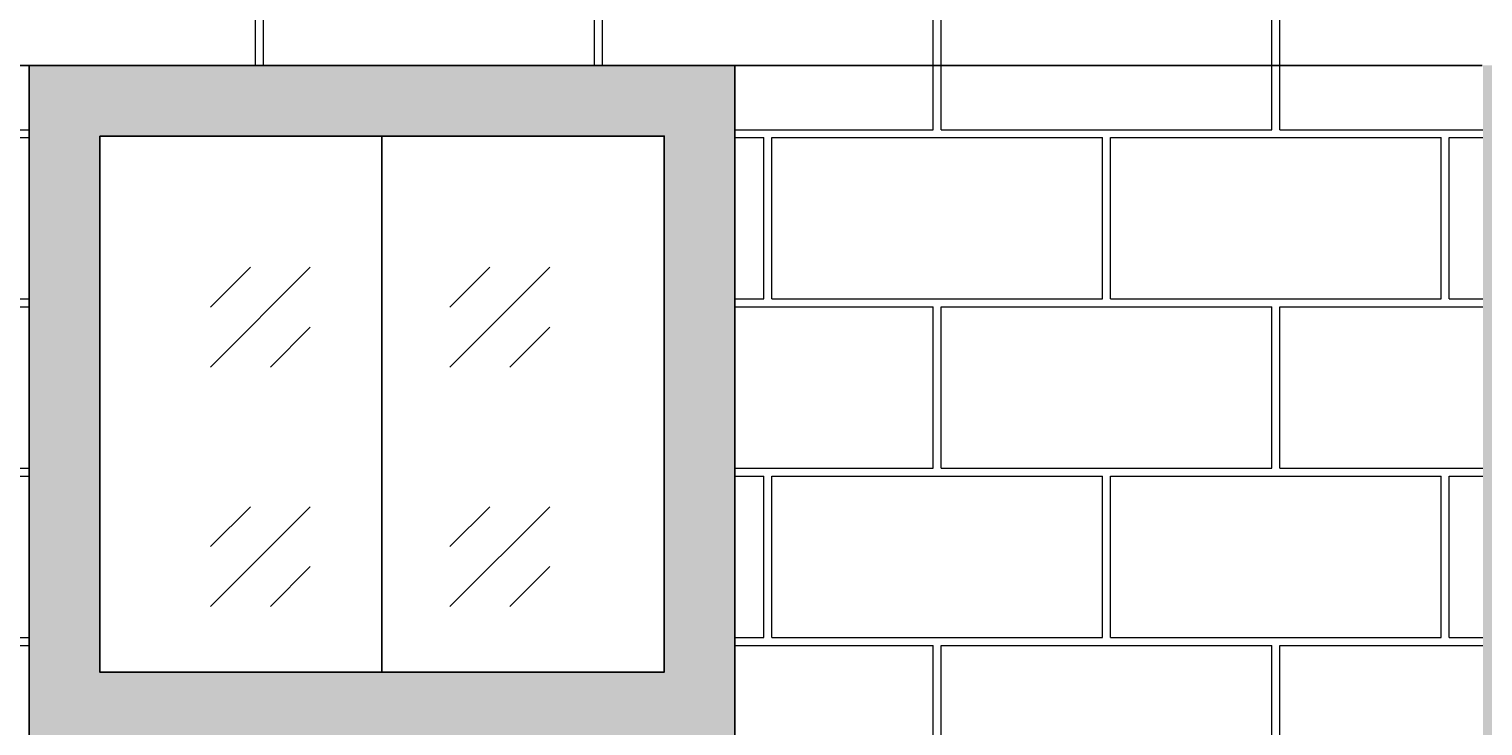
# Model space of a CAD drawing. Units: inches. Extents: x -301 to 715, y -607 to 364.
# Tile 134 of 141: x 310 to 413, y -440 to -391. Entities that reach past the tile are written whole.
import ezdxf

# ---------------------------------------------------------------- set-up
doc = ezdxf.new("R2010")
doc.units = ezdxf.units.IN
doc.header["$MEASUREMENT"] = 0
for name, color, linetype, lineweight in [('A-ANNO-DIMS', 2, 'Continuous', 18), ('A-ELEV-PATT', 4, 'Continuous', 13), ('A-GLAZ', 2, 'Continuous', 25)]:
    doc.layers.add(name, color=color, linetype=linetype, lineweight=lineweight)
doc.styles.get("Standard").update_dxf_attribs({"font": 'arial.ttf'})
doc.dimstyles.get("Standard").update_dxf_attribs({"dimtxt": 0.18, "dimasz": 0.18, "dimexe": 0.18, "dimexo": 0.0625, "dimgap": 0.09, "dimtad": 0, "dimtih": 1, "dimtoh": 1, "dimdec": 1, "dimzin": 0, "dimdsep": 46, "dimlunit": 4, "dimtxsty": 'Standard', "dimcen": 0.09, "dimclrd": 3, "dimclre": 4, "dimclrt": 6, "dimadec": 0, "dimazin": 0, "dimtfac": 1, "dimtdec": 1, "dimtofl": 0, "dimtmove": 0, "dimatfit": 3, "dimfxl": 1, "dimtfill": 2, "dimtfillclr": 51, "dimtolj": 1, "dimtzin": 0, "dimarcsym": 0})

# ---------------------------------------------------------------- blocks, each defined once
blk = doc.blocks.new('*D200')
at = {"layer": 'A-ANNO-DIMS', "color": 4, "lineweight": -2, "transparency": 16777216}
for p, q in [((412.96, -393.55), (121.93, -393.55)), ((412.96, -489.55), (121.93, -489.55))]:
    blk.add_line(p, q, dxfattribs=at)
at = {"layer": 'A-ANNO-DIMS', "color": 3, "lineweight": -2, "transparency": 16777216}
for p, q in [((122.11, -393.73), (122.11, -441.37)), ((122.11, -489.37), (122.11, -441.73))]:
    blk.add_line(p, q, dxfattribs=at)
at = {"layer": 'A-ANNO-DIMS', "color": 3, "transparency": 16777216}
for points in [[(122.08, -393.73), (122.14, -393.73), (122.11, -393.55)], [(122.08, -489.37), (122.14, -489.37), (122.11, -489.55)]]:
    blk.add_solid(points, dxfattribs=at)
at = {"layer": 'Defpoints', "color": 0, "transparency": 16777216}
for p in [(122.11, -393.55), (413.02, -393.55), (413.02, -489.55)]:
    blk.add_point(p, dxfattribs=at)
at = {"layer": 'A-ANNO-DIMS', "color": 6, "transparency": 16777216, "insert": (122.11, -441.55), "char_height": 0.18, "attachment_point": 5, "bg_fill": 1, "box_fill_scale": 1.25, "bg_fill_color": 51, "bg_fill_transparency": 0}
blk.add_mtext('\\A1;8\'-0"', dxfattribs=at)

msp = doc.modelspace()

# ---------------------------------------------------------------- hatches: boundary and pattern name
at = {"layer": 'A-ELEV-PATT'}
h = msp.add_hatch(color=256, dxfattribs=at)
h.dxf.hatch_style = 1
h.paths.add_polyline_path([(591.52, -363.55), (254.02, -363.55), (254.02, -369.55), (591.52, -369.55)])
h.paths.add_polyline_path([(461.02, -393.55), (413.02, -393.55), (413.02, -489.55), (461.02, -489.55)])
h.paths.add_polyline_path([(456.02, -398.55), (456.02, -484.55), (418.02, -484.55), (418.02, -398.55)], flags=16)
h.paths.add_polyline_path([(546.77, -393.55), (496.77, -393.55), (496.77, -441.55), (546.77, -441.55)])
h.paths.add_polyline_path([(501.77, -398.55), (541.77, -398.55), (541.77, -436.55), (501.77, -436.55)], flags=16)
h.paths.add_polyline_path([(360.02, -393.55), (310.02, -393.55), (310.02, -441.55), (360.02, -441.55)])
h.paths.add_polyline_path([(355.02, -398.55), (355.02, -436.55), (315.02, -436.55), (315.02, -398.55)], flags=16)
h = msp.add_hatch(dxfattribs=at)
h.set_pattern_fill('AR-B816C', color=256, scale=1.5)
h.set_pattern_definition([(0, (458.621, 9.325), (12, 12), [23.4375, -0.5625]), (0, (446.621, 9.887), (12, 12), [23.4375, -0.5625]), (90, (458.621, 9.325), (-12, 12), [-12.5625, 11.4375]), (90, (458.059, 9.325), (-12, 12), [-12.5625, 11.4375])])
h.paths.add_polyline_path([(254.02, -489.55), (413.02, -489.55), (413.02, -393.55), (461.02, -393.55), (461.02, -489.55), (591.52, -489.55), (591.52, -369.55), (254.02, -369.55)])
h.paths.add_polyline_path([(310.02, -393.55), (360.02, -393.55), (360.02, -441.55), (310.02, -441.55)], flags=16)
h.paths.add_polyline_path([(315.02, -398.55), (355.02, -398.55), (355.02, -436.55), (315.02, -436.55)], flags=0)
h.paths.add_polyline_path([(496.77, -393.55), (546.77, -393.55), (546.77, -441.55), (496.77, -441.55)], flags=16)
h.paths.add_polyline_path([(501.77, -398.55), (541.77, -398.55), (541.77, -436.55), (501.77, -436.55)], flags=0)
h = msp.add_hatch(dxfattribs=at)
h.set_pattern_fill('GOST_GLASS', color=256, scale=2)
h.set_pattern_definition([(45, (458.621, 9.325), (16.97056, -2e-15), [10, -14]), (45, (462.864, 9.325), (16.97056, -2e-15), [4, -20]), (45, (458.621, 13.567), (16.97056, -2e-15), [4, -20])])
h.paths.add_polyline_path([(335.02, -398.55), (315.02, -398.55), (315.02, -436.55), (335.02, -436.55)])
h.paths.add_polyline_path([(355.02, -398.55), (335.02, -398.55), (335.02, -436.55), (355.02, -436.55)])
h.paths.add_polyline_path([(521.77, -398.55), (501.77, -398.55), (501.77, -436.55), (521.77, -436.55)])
h.paths.add_polyline_path([(541.77, -398.55), (521.77, -398.55), (521.77, -436.55), (541.77, -436.55)])

# ---------------------------------------------------------------- linework, layer by layer
at = {"layer": 'A-GLAZ'}
msp.add_line((335.02, -398.55), (335.02, -436.55), dxfattribs=at)
for points in [[(310.02, -393.55), (360.02, -393.55), (360.02, -441.55), (310.02, -441.55)], [(315.02, -398.55), (355.02, -398.55), (355.02, -436.55), (315.02, -436.55)]]:
    msp.add_lwpolyline(points, close=True, dxfattribs=at)

# ---------------------------------------------------------------- dimensions: what is measured, and where the dimension line sits
at = {"layer": 'A-ANNO-DIMS'}
dim = msp.add_linear_dim(base=(122.11, -393.55), p1=(413.02, -489.55), p2=(413.02, -393.55), angle=90, dimstyle='Standard', override={"dimdec": 1, "dimlfac": 1, "dimrnd": 0, "dimzin": 1, "dimdsep": 46, "dimlunit": 4, "dimfrac": 2}, dxfattribs=at)
dim.commit()
dim.dimension.update_dxf_attribs({"geometry": '*D200', "text_midpoint": (122.11, -441.55)})

doc.saveas('drawing.dxf')
